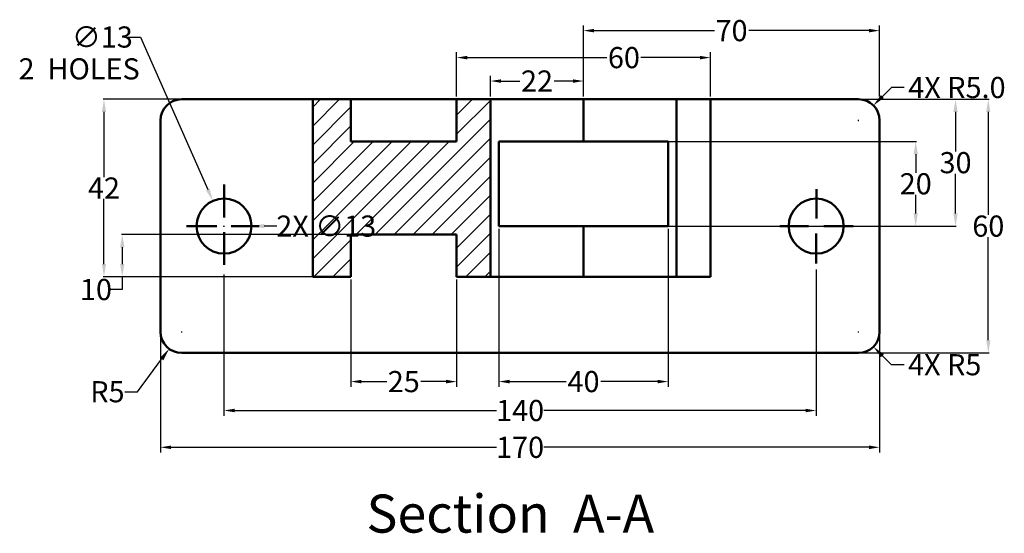
# Model space of a CAD drawing. Units: metres. Extents: x -2793 to -2360, y -31 to 491.
# Tile 3 of 4: x -2793 to -2560, y 370 to 491. Entities that reach past the tile are written whole.
import ezdxf

# ---------------------------------------------------------------- set-up
doc = ezdxf.new("R2010")
doc.units = ezdxf.units.M
for name, color, linetype, lineweight in [('M-DIMS', 2, 'Continuous', 25), ('M-HATC', 8, 'Continuous', 18), ('M-OUTL', 7, 'Continuous', 50), ('M-TEXT', 7, 'Continuous', 25)]:
    doc.layers.add(name, color=color, linetype=linetype, lineweight=lineweight)
doc.styles.get("Standard").update_dxf_attribs({"font": 'arial.ttf'})
doc.dimstyles.new('ISO-25', dxfattribs={"dimtxt": 2.5, "dimasz": 2.5, "dimexe": 1.25, "dimexo": 0.625, "dimtad": 0, "dimtxsty": 'Standard', "dimcen": 2.5, "dimadec": 0, "dimazin": 0, "dimtfac": 1, "dimtmove": 0, "dimatfit": 3, "dimfxl": 1, "dimarcsym": 0})
doc.dimstyles.get("Standard").update_dxf_attribs({"dimtxt": 5, "dimasz": 3, "dimexe": 0.18, "dimexo": 0.0625, "dimgap": 0.09, "dimtad": 0, "dimtih": 1, "dimtoh": 1, "dimdec": 0, "dimzin": 0, "dimdsep": 46, "dimtxsty": 'Standard', "dimcen": 0.09, "dimclrd": 254, "dimclre": 254, "dimadec": 0, "dimazin": 0, "dimtfac": 1, "dimtdec": 0, "dimtofl": 0, "dimtmove": 0, "dimatfit": 3, "dimfxl": 1, "dimtolj": 1, "dimtzin": 0, "dimarcsym": 0})

# ---------------------------------------------------------------- blocks, each defined once
blk = doc.blocks.new('*D1')
at = {"layer": 'Defpoints', "color": 0, "transparency": 16777216}
for p in [(-2744.87, 431.6), (-2604.87, 432.74), (-2604.87, 398.79)]:
    blk.add_point(p, dxfattribs=at)
at = {"layer": 'M-DIMS', "color": 0, "lineweight": -2, "transparency": 16777216}
for p, q in [((-2744.87, 430.97), (-2744.87, 397.54)), ((-2604.87, 432.11), (-2604.87, 397.54)), ((-2742.37, 398.79), (-2680.47, 398.79)), ((-2607.37, 398.79), (-2669.27, 398.79))]:
    blk.add_line(p, q, dxfattribs=at)
at = {"layer": 'M-DIMS', "color": 0, "transparency": 16777216}
for points in [[(-2742.37, 399.21), (-2742.37, 398.37), (-2744.87, 398.79)], [(-2607.37, 399.21), (-2607.37, 398.37), (-2604.87, 398.79)]]:
    blk.add_solid(points, dxfattribs=at)
at = {"layer": 'M-DIMS', "color": 0, "transparency": 16777216, "insert": (-2674.87, 398.79), "char_height": 2.5, "attachment_point": 5}
blk.add_mtext('{\\fTimes New Roman|b0|i0|c0|p18;\\H2x;\\C7;140}', dxfattribs=at)
blk = doc.blocks.new('*D2')
at = {"layer": 'Defpoints', "color": 0, "transparency": 16777216}
for p in [(-2714.87, 430.4), (-2689.87, 430.4), (-2689.87, 405.63)]:
    blk.add_point(p, dxfattribs=at)
at = {"layer": 'M-DIMS', "color": 0, "lineweight": -2, "transparency": 16777216}
for p, q in [((-2714.87, 429.77), (-2714.87, 404.38)), ((-2689.87, 429.77), (-2689.87, 404.38)), ((-2712.37, 405.63), (-2706.36, 405.63)), ((-2692.37, 405.63), (-2698.37, 405.63))]:
    blk.add_line(p, q, dxfattribs=at)
at = {"layer": 'M-DIMS', "color": 0, "transparency": 16777216}
for points in [[(-2712.37, 406.05), (-2712.37, 405.21), (-2714.87, 405.63)], [(-2692.37, 406.05), (-2692.37, 405.21), (-2689.87, 405.63)]]:
    blk.add_solid(points, dxfattribs=at)
at = {"layer": 'M-DIMS', "color": 0, "transparency": 16777216, "insert": (-2702.37, 405.63), "char_height": 2.5, "attachment_point": 5}
blk.add_mtext('{\\fTimes New Roman|b0|i0|c0|p18;\\H2x;\\C256;25}', dxfattribs=at)
blk = doc.blocks.new('*D3')
at = {"layer": 'Defpoints', "color": 0, "transparency": 16777216}
for p in [(-2681.87, 476.7), (-2681.87, 472.4), (-2659.87, 472.4)]:
    blk.add_point(p, dxfattribs=at)
at = {"layer": 'M-DIMS', "color": 0, "lineweight": -2, "transparency": 16777216}
for p, q in [((-2681.87, 473.02), (-2681.87, 477.95)), ((-2659.87, 473.02), (-2659.87, 477.95)), ((-2679.37, 476.7), (-2674.95, 476.7)), ((-2662.37, 476.7), (-2666.78, 476.7))]:
    blk.add_line(p, q, dxfattribs=at)
at = {"layer": 'M-DIMS', "color": 0, "transparency": 16777216}
for points in [[(-2679.37, 477.11), (-2679.37, 476.28), (-2681.87, 476.7)], [(-2662.37, 477.11), (-2662.37, 476.28), (-2659.87, 476.7)]]:
    blk.add_solid(points, dxfattribs=at)
at = {"layer": 'M-DIMS', "color": 0, "transparency": 16777216, "insert": (-2670.87, 476.7), "char_height": 2.5, "attachment_point": 5}
blk.add_mtext('{\\fTimes New Roman|b0|i0|c0|p18;\\H2x;\\C7;22}', dxfattribs=at)
blk = doc.blocks.new('*D4')
at = {"layer": 'Defpoints', "color": 0, "transparency": 16777216}
for p in [(-2689.87, 482.24), (-2689.87, 472.4), (-2629.87, 472.4)]:
    blk.add_point(p, dxfattribs=at)
at = {"layer": 'M-DIMS', "color": 0, "lineweight": -2, "transparency": 16777216}
for p, q in [((-2689.87, 473.02), (-2689.87, 483.49)), ((-2687.37, 482.24), (-2654.35, 482.24)), ((-2632.37, 482.24), (-2646.3, 482.24)), ((-2629.87, 473.02), (-2629.87, 483.49))]:
    blk.add_line(p, q, dxfattribs=at)
at = {"layer": 'M-DIMS', "color": 0, "transparency": 16777216}
for points in [[(-2687.37, 482.65), (-2687.37, 481.82), (-2689.87, 482.24)], [(-2632.37, 482.65), (-2632.37, 481.82), (-2629.87, 482.24)]]:
    blk.add_solid(points, dxfattribs=at)
at = {"layer": 'M-DIMS', "color": 0, "transparency": 16777216, "insert": (-2650.32, 482.24), "char_height": 2.5, "attachment_point": 5}
blk.add_mtext('{\\fTimes New Roman|b0|i0|c0|p18;\\H2x;\\C7;60}', dxfattribs=at)
blk = doc.blocks.new('*D5')
at = {"layer": 'Defpoints', "color": 0, "transparency": 16777216}
for p in [(-2659.87, 488.62), (-2659.87, 472.4), (-2589.87, 472.4)]:
    blk.add_point(p, dxfattribs=at)
at = {"layer": 'M-DIMS', "color": 0, "lineweight": -2, "transparency": 16777216}
for p, q in [((-2659.87, 473.02), (-2659.87, 489.87)), ((-2589.87, 473.02), (-2589.87, 489.87)), ((-2657.37, 488.62), (-2628.92, 488.62)), ((-2592.37, 488.62), (-2620.82, 488.62))]:
    blk.add_line(p, q, dxfattribs=at)
at = {"layer": 'M-DIMS', "color": 0, "transparency": 16777216}
for points in [[(-2657.37, 489.04), (-2657.37, 488.2), (-2659.87, 488.62)], [(-2592.37, 489.04), (-2592.37, 488.2), (-2589.87, 488.62)]]:
    blk.add_solid(points, dxfattribs=at)
at = {"layer": 'M-DIMS', "color": 0, "transparency": 16777216, "insert": (-2624.87, 488.62), "char_height": 2.5, "attachment_point": 5}
blk.add_mtext('{\\fTimes New Roman|b0|i0|c0|p18;\\H2x;\\C7;70}', dxfattribs=at)
blk = doc.blocks.new('*D6')
at = {"layer": 'Defpoints', "color": 0, "transparency": 16777216}
for p in [(-2679.87, 442.4), (-2639.87, 442.4), (-2639.87, 405.63)]:
    blk.add_point(p, dxfattribs=at)
at = {"layer": 'M-DIMS', "color": 0, "lineweight": -2, "transparency": 16777216}
for p, q in [((-2679.87, 441.77), (-2679.87, 404.38)), ((-2639.87, 441.77), (-2639.87, 404.38)), ((-2677.37, 405.63), (-2663.99, 405.63)), ((-2642.37, 405.63), (-2655.74, 405.63))]:
    blk.add_line(p, q, dxfattribs=at)
at = {"layer": 'M-DIMS', "color": 0, "transparency": 16777216}
for points in [[(-2677.37, 406.05), (-2677.37, 405.21), (-2679.87, 405.63)], [(-2642.37, 406.05), (-2642.37, 405.21), (-2639.87, 405.63)]]:
    blk.add_solid(points, dxfattribs=at)
at = {"layer": 'M-DIMS', "color": 0, "transparency": 16777216, "insert": (-2659.87, 405.63), "char_height": 2.5, "attachment_point": 5}
blk.add_mtext('{\\fTimes New Roman|b0|i0|c0|p18;\\H2x;\\C256;40}', dxfattribs=at)
blk = doc.blocks.new('*D7')
at = {"layer": 'Defpoints', "color": 0, "transparency": 16777216}
for p in [(-2759.87, 417.4), (-2589.87, 417.4), (-2589.87, 390.09)]:
    blk.add_point(p, dxfattribs=at)
at = {"layer": 'M-DIMS', "color": 0, "lineweight": -2, "transparency": 16777216}
for p, q in [((-2759.87, 416.77), (-2759.87, 388.84)), ((-2589.87, 416.77), (-2589.87, 388.84)), ((-2757.37, 390.09), (-2680.47, 390.09)), ((-2592.37, 390.09), (-2669.27, 390.09))]:
    blk.add_line(p, q, dxfattribs=at)
at = {"layer": 'M-DIMS', "color": 0, "transparency": 16777216}
for points in [[(-2757.37, 390.51), (-2757.37, 389.67), (-2759.87, 390.09)], [(-2592.37, 390.51), (-2592.37, 389.67), (-2589.87, 390.09)]]:
    blk.add_solid(points, dxfattribs=at)
at = {"layer": 'M-DIMS', "color": 0, "transparency": 16777216, "insert": (-2674.87, 390.09), "char_height": 2.5, "attachment_point": 5}
blk.add_mtext('{\\fTimes New Roman|b0|i0|c0|p18;\\H2x;\\C256;170}', dxfattribs=at)
blk = doc.blocks.new('*D8')
at = {"layer": 'Defpoints', "color": 0, "transparency": 16777216}
for p in [(-2639.87, 462.4), (-2639.87, 442.4), (-2581.34, 442.4)]:
    blk.add_point(p, dxfattribs=at)
at = {"layer": 'M-DIMS', "color": 0, "lineweight": -2, "transparency": 16777216}
for p, q in [((-2639.81, 462.4), (-2581.16, 462.4)), ((-2581.34, 459.4), (-2581.34, 455.03)), ((-2581.34, 445.4), (-2581.34, 449.76)), ((-2639.81, 442.4), (-2581.16, 442.4))]:
    blk.add_line(p, q, dxfattribs=at)
at = {"layer": 'M-DIMS', "color": 0, "transparency": 16777216}
for points in [[(-2581.84, 459.4), (-2580.84, 459.4), (-2581.34, 462.4)], [(-2581.84, 445.4), (-2580.84, 445.4), (-2581.34, 442.4)]]:
    blk.add_solid(points, dxfattribs=at)
at = {"layer": 'M-DIMS', "color": 0, "transparency": 16777216, "insert": (-2581.34, 452.4), "char_height": 5, "attachment_point": 5}
blk.add_mtext('\\A1;{\\fTimes New Roman|b0|i0|c0|p18;20}', dxfattribs=at)
blk = doc.blocks.new('*D9')
at = {"layer": 'Defpoints', "color": 0, "transparency": 16777216}
for p in [(-2604.87, 472.4), (-2571.92, 472.4), (-2604.87, 442.4)]:
    blk.add_point(p, dxfattribs=at)
at = {"layer": 'M-DIMS', "color": 0, "lineweight": -2, "transparency": 16777216}
for p, q in [((-2604.81, 472.4), (-2571.74, 472.4)), ((-2571.92, 469.4), (-2571.92, 460.03)), ((-2571.92, 445.4), (-2571.92, 454.76)), ((-2604.81, 442.4), (-2571.74, 442.4))]:
    blk.add_line(p, q, dxfattribs=at)
at = {"layer": 'M-DIMS', "color": 0, "transparency": 16777216}
for points in [[(-2572.42, 469.4), (-2571.42, 469.4), (-2571.92, 472.4)], [(-2572.42, 445.4), (-2571.42, 445.4), (-2571.92, 442.4)]]:
    blk.add_solid(points, dxfattribs=at)
at = {"layer": 'M-DIMS', "color": 0, "transparency": 16777216, "insert": (-2571.92, 457.4), "char_height": 5, "attachment_point": 5}
blk.add_mtext('\\A1;{\\fTimes New Roman|b0|i0|c0|p18;30}', dxfattribs=at)
blk = doc.blocks.new('*D10')
at = {"layer": 'Defpoints', "color": 0, "transparency": 16777216}
for p in [(-2594.72, 472.39), (-2594.87, 412.4), (-2564.17, 412.4)]:
    blk.add_point(p, dxfattribs=at)
at = {"layer": 'M-DIMS', "color": 0, "lineweight": -2, "transparency": 16777216}
for p, q in [((-2594.65, 472.39), (-2563.99, 472.39)), ((-2564.17, 469.39), (-2564.17, 445.03)), ((-2564.17, 415.4), (-2564.17, 439.76)), ((-2594.81, 412.4), (-2563.99, 412.4))]:
    blk.add_line(p, q, dxfattribs=at)
at = {"layer": 'M-DIMS', "color": 0, "transparency": 16777216}
for points in [[(-2564.67, 469.39), (-2563.67, 469.39), (-2564.17, 472.39)], [(-2564.67, 415.4), (-2563.67, 415.4), (-2564.17, 412.4)]]:
    blk.add_solid(points, dxfattribs=at)
at = {"layer": 'M-DIMS', "color": 0, "transparency": 16777216, "insert": (-2564.17, 442.4), "char_height": 5, "attachment_point": 5}
blk.add_mtext('\\A1;{\\fTimes New Roman|b0|i0|c0|p18;60}', dxfattribs=at)
blk = doc.blocks.new('*D11')
at = {"layer": 'Defpoints', "color": 0, "transparency": 16777216}
for p in [(-2714.87, 440.4), (-2768.93, 430.4), (-2714.87, 430.4)]:
    blk.add_point(p, dxfattribs=at)
at = {"layer": 'M-DIMS', "color": 0, "lineweight": -2, "transparency": 16777216}
for p, q in [((-2714.93, 440.4), (-2769.11, 440.4)), ((-2768.93, 437.4), (-2768.93, 433.4)), ((-2714.93, 430.4), (-2769.11, 430.4)), ((-2768.93, 430.4), (-2768.93, 427.4)), ((-2768.93, 427.4), (-2771.93, 427.4))]:
    blk.add_line(p, q, dxfattribs=at)
at = {"layer": 'M-DIMS', "color": 0, "transparency": 16777216}
for points in [[(-2769.43, 437.4), (-2768.43, 437.4), (-2768.93, 440.4)], [(-2769.43, 433.4), (-2768.43, 433.4), (-2768.93, 430.4)]]:
    blk.add_solid(points, dxfattribs=at)
at = {"layer": 'M-DIMS', "color": 0, "transparency": 16777216, "insert": (-2775.14, 427.4), "char_height": 5, "attachment_point": 5}
blk.add_mtext('\\A1;{\\fTimes New Roman|b0|i0|c0|p18;10}', dxfattribs=at)
blk = doc.blocks.new('*D12')
at = {"layer": 'Defpoints', "color": 0, "transparency": 16777216}
for p in [(-2723.87, 472.4), (-2773.25, 430.4), (-2723.87, 430.4)]:
    blk.add_point(p, dxfattribs=at)
at = {"layer": 'M-DIMS', "color": 0, "lineweight": -2, "transparency": 16777216}
for p, q in [((-2723.93, 472.4), (-2773.43, 472.4)), ((-2773.25, 469.4), (-2773.25, 453.99)), ((-2773.25, 433.4), (-2773.25, 448.81)), ((-2723.93, 430.4), (-2773.43, 430.4))]:
    blk.add_line(p, q, dxfattribs=at)
at = {"layer": 'M-DIMS', "color": 0, "transparency": 16777216}
for points in [[(-2773.75, 469.4), (-2772.75, 469.4), (-2773.25, 472.4)], [(-2773.75, 433.4), (-2772.75, 433.4), (-2773.25, 430.4)]]:
    blk.add_solid(points, dxfattribs=at)
at = {"layer": 'M-DIMS', "color": 0, "transparency": 16777216, "insert": (-2773.25, 451.4), "char_height": 5, "attachment_point": 5}
blk.add_mtext('\\A1;{\\fTimes New Roman|b0|i0|c0|p18;42}', dxfattribs=at)
blk = doc.blocks.new('*D13')
at = {"layer": 'Defpoints', "color": 0, "transparency": 16777216}
for p in [(-2747.49, 448.34), (-2742.24, 436.45)]:
    blk.add_point(p, dxfattribs=at)
at = {"layer": 'M-DIMS', "color": 0, "lineweight": -2, "transparency": 16777216}
for p, q in [((-2767.61, 487.11), (-2764.61, 487.11)), ((-2764.61, 487.11), (-2748.7, 451.09)), ((-2744.96, 442.4), (-2744.78, 442.4)), ((-2744.87, 442.31), (-2744.87, 442.49))]:
    blk.add_line(p, q, dxfattribs=at)
at = {"layer": 'M-DIMS', "color": 0, "transparency": 16777216}
blk.add_solid([(-2748.25, 451.29), (-2749.16, 450.89), (-2747.49, 448.34)], dxfattribs=at)
at = {"layer": 'M-DIMS', "color": 0, "transparency": 16777216, "insert": (-2773.62, 487.11), "char_height": 5, "attachment_point": 5}
blk.add_mtext('\\A1;{\\fTimes New Roman|b0|i0|c0|p18;∅13}', dxfattribs=at)
blk = doc.blocks.new('*D14')
at = {"layer": 'Defpoints', "color": 0, "transparency": 16777216}
for p in [(-2754.87, 417.4), (-2757.83, 413.37)]:
    blk.add_point(p, dxfattribs=at)
at = {"layer": 'M-DIMS', "color": 0, "lineweight": -2, "transparency": 16777216}
for p, q in [((-2754.96, 417.4), (-2754.78, 417.4)), ((-2754.87, 417.31), (-2754.87, 417.49)), ((-2765.29, 403.23), (-2759.61, 410.95)), ((-2768.34, 403.23), (-2765.29, 403.23))]:
    blk.add_line(p, q, dxfattribs=at)
at = {"layer": 'M-DIMS', "color": 0, "transparency": 16777216}
blk.add_solid([(-2760.01, 411.25), (-2759.21, 410.66), (-2757.83, 413.37)], dxfattribs=at)
at = {"layer": 'M-DIMS', "color": 0, "transparency": 16777216, "insert": (-2772.43, 403.23), "char_height": 5, "attachment_point": 5}
blk.add_mtext('\\A1;{\\fTimes New Roman|b0|i0|c0|p18;R5}', dxfattribs=at)
blk = doc.blocks.new('*D66')
at = {"layer": 'Defpoints', "color": 0, "transparency": 16777216}
for p in [(-2751.37, 442.4), (-2738.37, 442.4)]:
    blk.add_point(p, dxfattribs=at)
at = {"layer": 'M-DIMS', "color": 254, "lineweight": -2, "transparency": 16777216}
for p, q in [((-2744.96, 442.4), (-2744.78, 442.4)), ((-2744.87, 442.31), (-2744.87, 442.49)), ((-2732.37, 442.4), (-2735.37, 442.4))]:
    blk.add_line(p, q, dxfattribs=at)
at = {"layer": 'M-DIMS', "color": 254, "transparency": 16777216}
blk.add_solid([(-2735.37, 442.9), (-2735.37, 441.9), (-2738.37, 442.4)], dxfattribs=at)
at = {"layer": 'M-DIMS', "color": 0, "transparency": 16777216, "insert": (-2720.7, 442.4), "char_height": 5, "attachment_point": 5}
blk.add_mtext('\\A1;2X ∅13', dxfattribs=at)
blk = doc.blocks.new('*D67')
at = {"layer": 'Defpoints', "color": 0, "transparency": 16777216}
for p in [(-2594.87, 417.4), (-2591.33, 413.86)]:
    blk.add_point(p, dxfattribs=at)
at = {"layer": 'M-DIMS', "color": 254, "lineweight": -2, "transparency": 16777216}
for p, q in [((-2594.96, 417.4), (-2594.78, 417.4)), ((-2594.87, 417.31), (-2594.87, 417.49)), ((-2587.09, 409.62), (-2589.21, 411.74)), ((-2584.09, 409.62), (-2587.09, 409.62))]:
    blk.add_line(p, q, dxfattribs=at)
at = {"layer": 'M-DIMS', "color": 254, "transparency": 16777216}
blk.add_solid([(-2588.86, 412.09), (-2589.56, 411.39), (-2591.33, 413.86)], dxfattribs=at)
at = {"layer": 'M-DIMS', "color": 0, "transparency": 16777216, "insert": (-2574.48, 409.62), "char_height": 5, "attachment_point": 5}
blk.add_mtext('\\A1;4X R5', dxfattribs=at)
blk = doc.blocks.new('*D74')
at = {"layer": 'Defpoints', "color": 0, "transparency": 16777216}
for p in [(-2591.33, 470.93), (-2594.87, 467.4)]:
    blk.add_point(p, dxfattribs=at)
at = {"layer": 'M-DIMS', "color": 254, "lineweight": -2, "transparency": 16777216}
for p, q in [((-2587.09, 475.17), (-2589.21, 473.05)), ((-2584.09, 475.17), (-2587.09, 475.17)), ((-2594.96, 467.4), (-2594.78, 467.4)), ((-2594.87, 467.31), (-2594.87, 467.49))]:
    blk.add_line(p, q, dxfattribs=at)
at = {"layer": 'M-DIMS', "color": 254, "transparency": 16777216}
blk.add_solid([(-2589.56, 473.41), (-2588.86, 472.7), (-2591.33, 470.93)], dxfattribs=at)
at = {"layer": 'M-DIMS', "color": 0, "transparency": 16777216, "insert": (-2571.59, 475.17), "char_height": 5, "attachment_point": 5}
blk.add_mtext('\\A1;4X R5.0', dxfattribs=at)

msp = doc.modelspace()

# ---------------------------------------------------------------- hatches: boundary and pattern name
at = {"layer": 'M-HATC'}
h = msp.add_hatch(dxfattribs=at)
h.set_pattern_fill('ANSI31', color=256)
h.set_pattern_definition([(45, (-6180.561, -1185.6038), (-2.245064, 2.245064), [])])
h.paths.add_polyline_path([(-2681.868, 472.397), (-2689.868, 472.397), (-2689.868, 462.397), (-2714.868, 462.397), (-2714.868, 472.397), (-2723.868, 472.397), (-2723.868, 430.397), (-2714.868, 430.397), (-2714.868, 440.397), (-2689.868, 440.397), (-2689.868, 430.397), (-2681.868, 430.397)])

# ---------------------------------------------------------------- linework, layer by layer
at = {"layer": 'M-OUTL'}
for p, q in [((-2594.868, 472.397), (-2754.868, 472.397)), ((-2723.868, 430.397), (-2723.868, 472.397)), ((-2689.868, 472.397), (-2714.868, 472.397)), ((-2714.868, 472.397), (-2714.868, 462.397)), ((-2689.868, 462.397), (-2689.868, 472.397)), ((-2681.868, 430.397), (-2681.868, 472.397)), ((-2659.868, 462.397), (-2659.868, 472.397)), ((-2637.868, 430.397), (-2637.868, 472.397)), ((-2629.868, 430.397), (-2629.868, 472.397)), ((-2759.868, 467.397), (-2759.868, 417.397)), ((-2589.868, 417.397), (-2589.868, 467.397)), ((-2689.868, 462.397), (-2714.868, 462.397)), ((-2639.868, 462.397), (-2679.868, 462.397)), ((-2679.868, 462.397), (-2679.868, 442.397)), ((-2639.868, 462.397), (-2679.868, 462.397)), ((-2639.868, 442.397), (-2639.868, 462.397)), ((-2744.868, 452.235), (-2744.868, 444.461)), ((-2604.787, 451.159), (-2604.819, 444.183)), ((-2753.719, 442.397), (-2746.575, 442.397)), ((-2743.16, 442.397), (-2736.525, 442.397)), ((-2679.868, 442.397), (-2659.868, 442.397)), ((-2659.868, 430.397), (-2659.868, 442.397)), ((-2659.868, 442.397), (-2639.868, 442.397)), ((-2613.486, 442.397), (-2606.655, 442.397)), ((-2603.081, 442.397), (-2596.088, 442.397)), ((-2744.868, 440.984), (-2744.868, 433.21)), ((-2689.868, 440.397), (-2714.868, 440.397)), ((-2714.868, 440.397), (-2714.868, 430.397)), ((-2689.868, 430.397), (-2689.868, 440.397)), ((-2604.835, 440.61), (-2604.868, 433.574)), ((-2714.868, 430.397), (-2723.868, 430.397)), ((-2629.868, 430.397), (-2689.868, 430.397)), ((-2754.868, 412.397), (-2594.868, 412.397))]:
    msp.add_line(p, q, dxfattribs=at)
for centre in [(-2744.868, 442.397), (-2604.868, 442.397)]:
    msp.add_circle(centre, 6.5, dxfattribs=at)
for centre, start, end in [((-2754.868, 467.397), 90, 180), ((-2594.868, 467.397), 0, 90), ((-2754.868, 417.397), 180, 270), ((-2594.868, 417.397), 270, 0)]:
    msp.add_arc(centre, 5, start, end, dxfattribs=at)

# ---------------------------------------------------------------- texts
at = {"layer": 'M-TEXT', "attachment_point": 1}
for s, width, insert, char_height in [('{\\fTimes New Roman|b0|i0|c0|p18;2  HOLES}', 37.90167, (-2793.445, 482.08), 5), ('{\\fTimes New Roman|b0|i0|c0|p18;Section  A-A}', 97.45826, (-2711.183, 378.912), 9)]:
    msp.add_mtext_dynamic_manual_height_columns(s, width=width, gutter_width=12.5, heights=[0], dxfattribs=dict(at, insert=insert, char_height=char_height))

# ---------------------------------------------------------------- dimensions: what is measured, and where the dimension line sits
at = {"layer": 'M-DIMS'}
for base, p1, p2, text, picture, middle in [((-2659.868, 488.619), (-2589.868, 472.397), (-2659.868, 472.397), '{\\fTimes New Roman|b0|i0|c0|p18;\\H2x;\\C7;<>}', '*D5', (-2624.868, 488.619)), ((-2689.868, 482.236), (-2629.868, 472.397), (-2689.868, 472.397), '{\\fTimes New Roman|b0|i0|c0|p18;\\H2x;\\C7;<>}', '*D4', (-2650.322, 482.236)), ((-2681.868, 476.698), (-2659.868, 472.397), (-2681.868, 472.397), '{\\fTimes New Roman|b0|i0|c0|p18;\\H2x;\\C7;<>}', '*D3', (-2670.868, 476.698)), ((-2639.868, 405.631), (-2679.868, 442.397), (-2639.868, 442.397), '{\\fTimes New Roman|b0|i0|c0|p18;\\H2x;\\C256;<>}', '*D6', (-2659.868, 405.631)), ((-2604.868, 398.79), (-2744.868, 431.598), (-2604.868, 432.739), '{\\fTimes New Roman|b0|i0|c0|p18;\\H2x;\\C7;<>}', '*D1', (-2674.868, 398.79)), ((-2589.868, 390.092), (-2759.868, 417.397), (-2589.868, 417.397), '{\\fTimes New Roman|b0|i0|c0|p18;\\H2x;\\C256;<>}', '*D7', (-2674.868, 390.092))]:
    dim = msp.add_linear_dim(base=base, p1=p1, p2=p2, text=text, dimstyle='ISO-25', override={"dimclrd": 0, "dimclre": 0, "dimclrt": 0}, dxfattribs=at)
    dim.commit()
    dim.dimension.update_dxf_attribs({"geometry": picture, "text_midpoint": middle, "dimtype": 160})
for p1, p2, text, override, picture, middle in [((-2742.243, 436.45), (-2747.493, 448.343), '{\\fTimes New Roman|b0|i0|c0|p18;<>}', {"dimclrd": 0, "dimclre": 0, "dimclrt": 0}, '*D13', (-2773.616, 487.112)), ((-2751.368, 442.396), (-2738.368, 442.397), '2X <>', {"dimdec": 0, "dimlfac": 1, "dimrnd": 0, "dimzin": 0, "dimdsep": 46, "dimlunit": 2}, '*D66', (-2732.368, 442.397))]:
    dim = msp.add_diameter_dim_2p(p1=p1, p2=p2, text=text, dimstyle='Standard', override=override, dxfattribs=at)
    dim.commit()
    dim.dimension.update_dxf_attribs({"geometry": picture, "text_midpoint": middle, "dimtype": 163})
for center, mpoint, override, picture, middle in [((-2594.868, 467.397), (-2591.332, 470.932), {"dimdec": 1, "dimlfac": 1, "dimrnd": 0, "dimzin": 0, "dimdsep": 46, "dimlunit": 2}, '*D74', (-2571.591, 475.174)), ((-2594.868, 417.397), (-2591.332, 413.861), {"dimdec": 0, "dimlfac": 1, "dimrnd": 0, "dimzin": 0, "dimdsep": 46, "dimlunit": 2}, '*D67', (-2574.477, 409.618))]:
    dim = msp.add_radius_dim(center=center, mpoint=mpoint, text='4X <>', dimstyle='Standard', override=override, dxfattribs=at)
    dim.commit()
    dim.dimension.update_dxf_attribs({"geometry": picture, "text_midpoint": middle})
for base, p1, p2, picture, middle in [((-2773.245, 430.397), (-2723.868, 472.397), (-2723.868, 430.397), '*D12', (-2773.245, 451.397)), ((-2564.174, 412.397), (-2594.717, 472.394), (-2594.868, 412.397), '*D10', (-2564.174, 442.395)), ((-2581.341, 442.397), (-2639.868, 462.397), (-2639.868, 442.397), '*D8', (-2581.341, 452.397)), ((-2768.927, 430.397), (-2714.868, 440.397), (-2714.868, 430.397), '*D11', (-2775.144, 427.397))]:
    dim = msp.add_linear_dim(base=base, p1=p1, p2=p2, angle=90, text='{\\fTimes New Roman|b0|i0|c0|p18;<>}', dimstyle='Standard', override={"dimclrd": 0, "dimclre": 0, "dimclrt": 0}, dxfattribs=at)
    dim.commit()
    dim.dimension.update_dxf_attribs({"geometry": picture, "text_midpoint": middle})
dim = msp.add_linear_dim(base=(-2571.92, 472.397), p1=(-2604.868, 442.397), p2=(-2604.868, 472.397), angle=90, text='{\\fTimes New Roman|b0|i0|c0|p18;<>}', dimstyle='Standard', override={"dimclrd": 0, "dimclre": 0, "dimclrt": 0}, dxfattribs=at)
dim.commit()
dim.dimension.update_dxf_attribs({"geometry": '*D9', "text_midpoint": (-2571.92, 457.397), "dimtype": 160})
dim = msp.add_linear_dim(base=(-2689.868, 405.631), p1=(-2714.868, 430.397), p2=(-2689.868, 430.397), text='{\\fTimes New Roman|b0|i0|c0|p18;\\H2x;\\C256;<>}', dimstyle='ISO-25', override={"dimclrd": 0, "dimclre": 0, "dimclrt": 0}, dxfattribs=at)
dim.commit()
dim.dimension.update_dxf_attribs({"geometry": '*D2', "text_midpoint": (-2702.368, 405.631)})
dim = msp.add_radius_dim(center=(-2754.868, 417.397), mpoint=(-2757.83, 413.369), text='{\\fTimes New Roman|b0|i0|c0|p18;<>}', dimstyle='Standard', override={"dimclrd": 0, "dimclre": 0, "dimclrt": 0}, dxfattribs=at)
dim.commit()
dim.dimension.update_dxf_attribs({"geometry": '*D14', "text_midpoint": (-2772.431, 403.226), "dimtype": 164})

doc.saveas('drawing.dxf')
